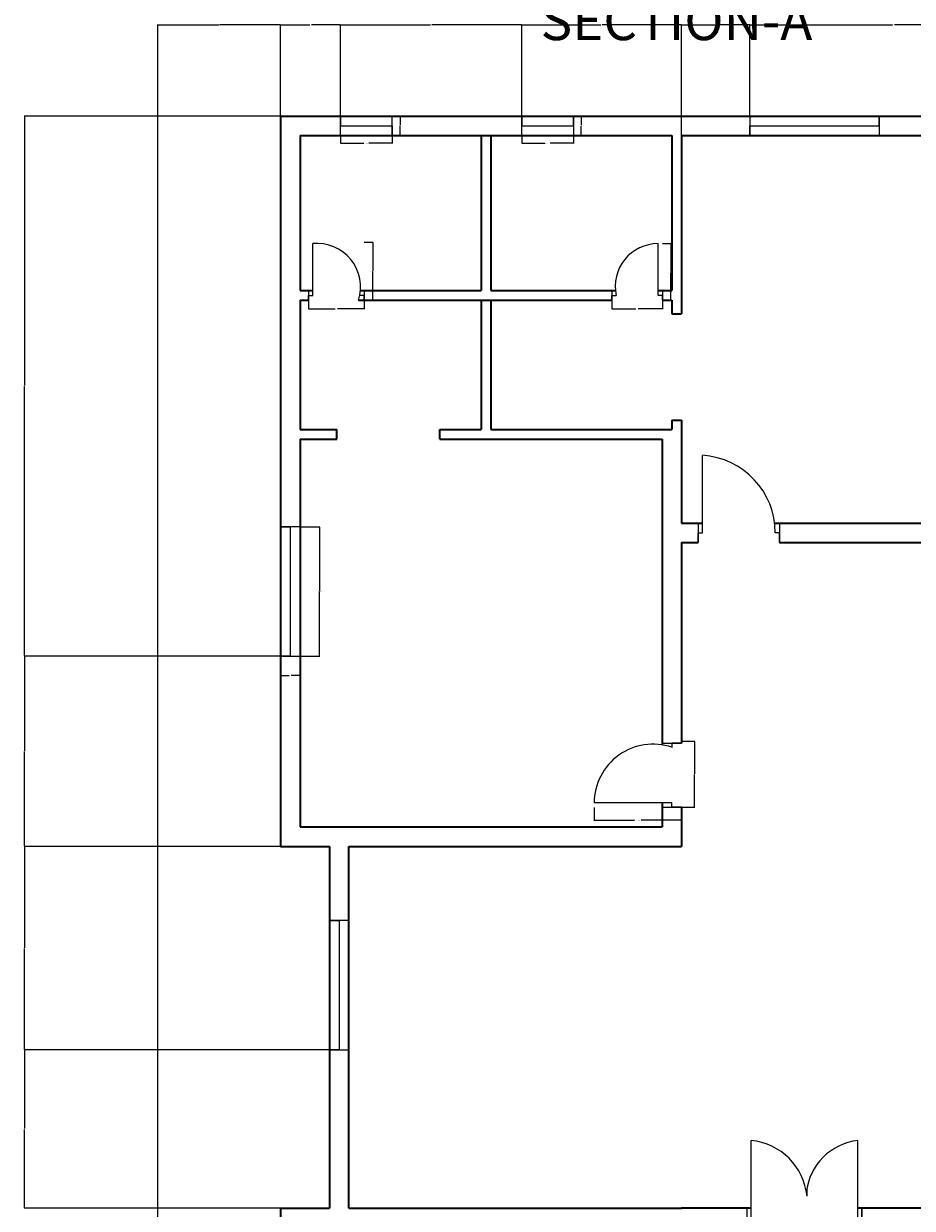
# Model space of a CAD drawing. Units: inches. Extents: x 1824 to 3509, y 619 to 2294.
# Tile 10 of 12: x 2571 to 2983, y 1115 to 1665. Entities that reach past the tile are written whole.
import ezdxf

# ---------------------------------------------------------------- set-up
doc = ezdxf.new("R2010")
doc.units = ezdxf.units.IN
for name, color, linetype, lineweight in [('A-ANNO-DIMS', 2, 'Continuous', 18), ('A-ANNO-TEXT', 7, 'Continuous', 25), ('A-DOOR', 3, 'Continuous', 18), ('A-GLAZ', 4, 'Continuous', 18), ('A-WALL', 7, 'Continuous', 35)]:
    doc.layers.add(name, color=color, linetype=linetype, lineweight=lineweight)
doc.styles.get("Standard").update_dxf_attribs({"font": 'arial.ttf'})
doc.dimstyles.get("Standard").update_dxf_attribs({"dimtxt": 0.18, "dimasz": 0.18, "dimexe": 0.18, "dimexo": 0.0625, "dimgap": 0.09, "dimtad": 0, "dimtih": 1, "dimtoh": 1, "dimdec": 4, "dimzin": 0, "dimdsep": 46, "dimtxsty": 'Standard', "dimcen": 0.09, "dimadec": 0, "dimazin": 0, "dimtfac": 1, "dimtdec": 4, "dimtofl": 0, "dimtmove": 0, "dimatfit": 3, "dimfxl": 1, "dimtolj": 1, "dimtzin": 0, "dimarcsym": 0})

# ---------------------------------------------------------------- blocks, each defined once
blk = doc.blocks.new('DOOR-BATH-W-24')
for p, q in [((2, 2.25), (2, 26.25)), ((0, 4.5), (0, 0)), ((0, 0), (0, 2.25)), ((0, 2.25), (2, 2.25)), ((25.84, 2.25), (23.84, 2.25)), ((25.84, 4.5), (25.84, 0)), ((25.84, 0), (25.84, 2.25))]:
    blk.add_line(p, q)
blk.add_arc((4.03, 6.16), 20.2, 342.2542, 95.7568)
blk = doc.blocks.new('DOOR-BATH-C-24')
for p, q in [((21.44, 2.25), (21.44, 26.25)), ((0, 4.5), (0, 0)), ((0, 0), (0, 2.25)), ((0, 2.25), (2, 2.25)), ((23.44, 2.25), (21.44, 2.25)), ((23.44, 4.5), (23.44, 0)), ((23.44, 0), (23.44, 2.25))]:
    blk.add_line(p, q)
blk.add_arc((21.44, 6.38), 19.87, 90, 191.9846)
blk = doc.blocks.new('DOOR-BED-W-36')
for p, q in [((31.5, 29.8), (40.5, 29.8)), ((40.5, 29.8), (36, 29.8)), ((36, 29.8), (36, 27.8)), ((36, 2), (0, 2)), ((31.5, 0), (31.5, 0)), ((31.5, 0), (40.5, 0)), ((36, 0), (36, 2)), ((40.5, 0), (36, 0)), ((36, 0), (36, 0)), ((40.5, 0), (40.5, 0))]:
    blk.add_line(p, q)
blk.add_arc((27.25, 2), 27.25, 71.2585, 180)
blk = doc.blocks.new('DOOR-BED-C-36')
for p, q in [((2, 4.5), (2, 40.5)), ((0, 9), (0, 0)), ((37.83, 9), (37.83, 9)), ((37.83, 9), (37.83, 0)), ((0, 0), (0, 4.5)), ((0, 4.5), (2, 4.5)), ((37.83, 4.5), (35.83, 4.5)), ((37.83, 0), (37.83, 4.5))]:
    blk.add_line(p, q)
blk.add_arc((-0.24, 4.5), 36.07, 0, 86.4439)
blk = doc.blocks.new('DOOR-LOUNGE-PAIR')
for p, q in [((2, 4.5), (2, 40.5)), ((51.41, 4.5), (51.41, 40.5)), ((27.9, 14.63), (27.9, 18.05)), ((0, 9), (0, 0)), ((53.41, 0), (53.41, 9)), ((53.41, 9), (53.41, 4.5)), ((0, 0), (0, 4.5)), ((0, 4.5), (2, 4.5)), ((53.41, 4.5), (51.41, 4.5)), ((53.41, 4.5), (53.41, 4.5))]:
    blk.add_line(p, q)
for centre, radius, start, end in [((-0.78, 11.81), 28.82, 5.6014, 84.4566), ((54.5, 13.67), 27.01, 96.5732, 173.8895)]:
    blk.add_arc(centre, radius, start, end)
blk = doc.blocks.new('WIN-24')
for p, q in [((0, 0), (0, 9)), ((0, 9), (0, 4.5)), ((24, 0), (24, 9)), ((0, 4.5), (24, 4.5)), ((24, 4.5), (24, 0))]:
    blk.add_line(p, q)
blk = doc.blocks.new('WIN-60')
for p, q in [((0, 9), (0, 0)), ((60, 4.5), (60, 9)), ((60, 9), (60, 0)), ((0, 0), (0, 4.5)), ((0, 4.5), (60, 4.5))]:
    blk.add_line(p, q)
blk = doc.blocks.new('WIN-60-SIDE')
for p, q in [((9, 60), (0, 60)), ((0, 60), (4.5, 60)), ((4.5, 60), (4.5, 0)), ((4.5, 0), (0, 0)), ((0, 0), (9, 0))]:
    blk.add_line(p, q)
blk = doc.blocks.new('WIN-24-TOP')
for p, q in [((0, 0), (0, 9)), ((0, 9), (0, 4.5)), ((24, 4.5), (24, 9)), ((24, 9), (24, 0)), ((0, 4.5), (24, 4.5))]:
    blk.add_line(p, q)
blk = doc.blocks.new('*D32')
at = {"layer": 'A-ANNO-DIMS', "color": 0, "lineweight": -2, "transparency": 16777216}
for p, q in [((2717.54, 1613.04), (2717.54, 1609.32)), ((2741.54, 1613.04), (2741.54, 1609.32)), ((2717.72, 1609.5), (2728.42, 1609.5)), ((2741.36, 1609.5), (2730.65, 1609.5))]:
    blk.add_line(p, q, dxfattribs=at)
at = {"layer": 'A-ANNO-DIMS', "color": 0, "transparency": 16777216}
for points in [[(2717.72, 1609.53), (2717.72, 1609.47), (2717.54, 1609.5)], [(2741.36, 1609.53), (2741.36, 1609.47), (2741.54, 1609.5)]]:
    blk.add_solid(points, dxfattribs=at)
at = {"layer": 'Defpoints', "color": 0, "transparency": 16777216}
for p in [(2717.54, 1613.1), (2741.54, 1613.1), (2741.54, 1609.5)]:
    blk.add_point(p, dxfattribs=at)
at = {"layer": 'A-ANNO-DIMS', "color": 0, "transparency": 16777216, "insert": (2729.54, 1609.5), "char_height": 0.18, "attachment_point": 5}
blk.add_mtext('\\A1;WINDOW 24 TYP.', dxfattribs=at)
blk = doc.blocks.new('*D33')
at = {"layer": 'A-ANNO-DIMS', "color": 0, "lineweight": -2, "transparency": 16777216}
for p, q in [((2741.6, 1622.1), (2745.32, 1622.1)), ((2745.14, 1621.92), (2745.14, 1617.78)), ((2745.14, 1613.28), (2745.14, 1617.42)), ((2741.6, 1613.1), (2745.32, 1613.1))]:
    blk.add_line(p, q, dxfattribs=at)
at = {"layer": 'A-ANNO-DIMS', "color": 0, "transparency": 16777216}
for points in [[(2745.11, 1621.92), (2745.17, 1621.92), (2745.14, 1622.1)], [(2745.11, 1613.28), (2745.17, 1613.28), (2745.14, 1613.1)]]:
    blk.add_solid(points, dxfattribs=at)
at = {"layer": 'Defpoints', "color": 0, "transparency": 16777216}
for p in [(2741.54, 1622.1), (2745.14, 1622.1), (2741.54, 1613.1)]:
    blk.add_point(p, dxfattribs=at)
at = {"layer": 'A-ANNO-DIMS', "color": 0, "transparency": 16777216, "insert": (2745.14, 1617.6), "char_height": 0.18, "attachment_point": 5}
blk.add_mtext('\\A1;9 TYP.', dxfattribs=at)
blk = doc.blocks.new('*D44')
at = {"layer": 'A-ANNO-DIMS', "color": 0, "lineweight": -2, "transparency": 16777216}
for p, q in [((2698.79, 1431.44), (2707.91, 1431.44)), ((2707.73, 1431.26), (2707.73, 1401.62)), ((2707.73, 1371.62), (2707.73, 1401.26)), ((2698.79, 1371.44), (2707.91, 1371.44))]:
    blk.add_line(p, q, dxfattribs=at)
at = {"layer": 'A-ANNO-DIMS', "color": 0, "transparency": 16777216}
for points in [[(2707.7, 1431.26), (2707.76, 1431.26), (2707.73, 1431.44)], [(2707.7, 1371.62), (2707.76, 1371.62), (2707.73, 1371.44)]]:
    blk.add_solid(points, dxfattribs=at)
at = {"layer": 'Defpoints', "color": 0, "transparency": 16777216}
for p in [(2698.73, 1431.44), (2707.73, 1431.44), (2698.73, 1371.44)]:
    blk.add_point(p, dxfattribs=at)
at = {"layer": 'A-ANNO-DIMS', "color": 0, "transparency": 16777216, "insert": (2707.73, 1401.44), "char_height": 0.18, "attachment_point": 5}
blk.add_mtext('\\A1;SIDE WINDOW 60 TYP.', dxfattribs=at)
blk = doc.blocks.new('*D45')
at = {"layer": 'A-ANNO-DIMS', "color": 0, "lineweight": -2, "transparency": 16777216}
for p, q in [((2689.73, 1371.38), (2689.73, 1362.26)), ((2698.73, 1371.38), (2698.73, 1362.26)), ((2689.91, 1362.44), (2693.77, 1362.44)), ((2698.55, 1362.44), (2694.69, 1362.44))]:
    blk.add_line(p, q, dxfattribs=at)
at = {"layer": 'A-ANNO-DIMS', "color": 0, "transparency": 16777216}
for points in [[(2689.91, 1362.47), (2689.91, 1362.41), (2689.73, 1362.44)], [(2698.55, 1362.47), (2698.55, 1362.41), (2698.73, 1362.44)]]:
    blk.add_solid(points, dxfattribs=at)
at = {"layer": 'Defpoints', "color": 0, "transparency": 16777216}
for p in [(2689.73, 1371.44), (2698.73, 1371.44), (2698.73, 1362.44)]:
    blk.add_point(p, dxfattribs=at)
at = {"layer": 'A-ANNO-DIMS', "color": 0, "transparency": 16777216, "insert": (2694.23, 1362.44), "char_height": 0.18, "attachment_point": 5}
blk.add_mtext('\\A1;9 TYP.', dxfattribs=at)
blk = doc.blocks.new('*D56')
at = {"layer": 'A-ANNO-DIMS', "color": 0, "lineweight": -2, "transparency": 16777216}
for p, q in [((2728.54, 1563.53), (2732.69, 1563.53)), ((2732.51, 1563.35), (2732.51, 1550.25)), ((2732.51, 1536.78), (2732.51, 1549.88)), ((2728.54, 1536.6), (2732.69, 1536.6))]:
    blk.add_line(p, q, dxfattribs=at)
at = {"layer": 'A-ANNO-DIMS', "color": 0, "transparency": 16777216}
for points in [[(2732.48, 1563.35), (2732.54, 1563.35), (2732.51, 1563.53)], [(2732.48, 1536.78), (2732.54, 1536.78), (2732.51, 1536.6)]]:
    blk.add_solid(points, dxfattribs=at)
at = {"layer": 'Defpoints', "color": 0, "transparency": 16777216}
for p in [(2728.47, 1563.53), (2732.51, 1563.53), (2728.47, 1536.6)]:
    blk.add_point(p, dxfattribs=at)
at = {"layer": 'A-ANNO-DIMS', "color": 0, "transparency": 16777216, "insert": (2732.51, 1550.07), "char_height": 0.18, "attachment_point": 5}
blk.add_mtext('\\A1;BATH DOOR 27 TYP.', dxfattribs=at)
blk = doc.blocks.new('*D57')
at = {"layer": 'A-ANNO-DIMS', "color": 0, "lineweight": -2, "transparency": 16777216}
for p, q in [((2702.63, 1536.54), (2702.63, 1532.38)), ((2728.47, 1536.54), (2728.47, 1532.38)), ((2702.81, 1532.56), (2715.02, 1532.56)), ((2728.29, 1532.56), (2716.08, 1532.56))]:
    blk.add_line(p, q, dxfattribs=at)
at = {"layer": 'A-ANNO-DIMS', "color": 0, "transparency": 16777216}
for points in [[(2702.81, 1532.59), (2702.81, 1532.53), (2702.63, 1532.56)], [(2728.29, 1532.59), (2728.29, 1532.53), (2728.47, 1532.56)]]:
    blk.add_solid(points, dxfattribs=at)
at = {"layer": 'Defpoints', "color": 0, "transparency": 16777216}
for p in [(2702.63, 1536.6), (2728.47, 1536.6), (2728.47, 1532.56)]:
    blk.add_point(p, dxfattribs=at)
at = {"layer": 'A-ANNO-DIMS', "color": 0, "transparency": 16777216, "insert": (2715.55, 1532.56), "char_height": 0.18, "attachment_point": 5}
blk.add_mtext('\\A1;26 TYP.', dxfattribs=at)
blk = doc.blocks.new('*D58')
at = {"layer": 'A-ANNO-DIMS', "color": 0, "lineweight": -2, "transparency": 16777216}
for p, q in [((2866.92, 1562.85), (2870.97, 1562.85)), ((2870.79, 1562.67), (2870.79, 1549.91)), ((2870.79, 1536.78), (2870.79, 1549.54)), ((2866.92, 1536.6), (2870.97, 1536.6))]:
    blk.add_line(p, q, dxfattribs=at)
at = {"layer": 'A-ANNO-DIMS', "color": 0, "transparency": 16777216}
for points in [[(2870.76, 1562.67), (2870.82, 1562.67), (2870.79, 1562.85)], [(2870.76, 1536.78), (2870.82, 1536.78), (2870.79, 1536.6)]]:
    blk.add_solid(points, dxfattribs=at)
at = {"layer": 'Defpoints', "color": 0, "transparency": 16777216}
for p in [(2866.86, 1562.85), (2870.79, 1562.85), (2866.86, 1536.6)]:
    blk.add_point(p, dxfattribs=at)
at = {"layer": 'A-ANNO-DIMS', "color": 0, "transparency": 16777216, "insert": (2870.79, 1549.73), "char_height": 0.18, "attachment_point": 5}
blk.add_mtext('\\A1;BATH DOOR 26 TYP.', dxfattribs=at)
blk = doc.blocks.new('*D59')
at = {"layer": 'A-ANNO-DIMS', "color": 0, "lineweight": -2, "transparency": 16777216}
for p, q in [((2843.42, 1536.54), (2843.42, 1532.48)), ((2866.86, 1536.54), (2866.86, 1532.48)), ((2843.6, 1532.66), (2854.61, 1532.66)), ((2866.68, 1532.66), (2855.67, 1532.66))]:
    blk.add_line(p, q, dxfattribs=at)
at = {"layer": 'A-ANNO-DIMS', "color": 0, "transparency": 16777216}
for points in [[(2843.6, 1532.69), (2843.6, 1532.63), (2843.42, 1532.66)], [(2866.68, 1532.69), (2866.68, 1532.63), (2866.86, 1532.66)]]:
    blk.add_solid(points, dxfattribs=at)
at = {"layer": 'Defpoints', "color": 0, "transparency": 16777216}
for p in [(2843.42, 1536.6), (2866.86, 1536.6), (2866.86, 1532.66)]:
    blk.add_point(p, dxfattribs=at)
at = {"layer": 'A-ANNO-DIMS', "color": 0, "transparency": 16777216, "insert": (2855.14, 1532.66), "char_height": 0.18, "attachment_point": 5}
blk.add_mtext('\\A1;23 TYP.', dxfattribs=at)
blk = doc.blocks.new('*D60')
at = {"layer": 'A-ANNO-DIMS', "color": 0, "lineweight": -2, "transparency": 16777216}
for p, q in [((2835.23, 1301.2), (2835.23, 1295.01)), ((2875.73, 1301.2), (2875.73, 1295.01)), ((2835.41, 1295.19), (2853.86, 1295.19)), ((2875.55, 1295.19), (2857.1, 1295.19))]:
    blk.add_line(p, q, dxfattribs=at)
at = {"layer": 'A-ANNO-DIMS', "color": 0, "transparency": 16777216}
for points in [[(2835.41, 1295.22), (2835.41, 1295.16), (2835.23, 1295.19)], [(2875.55, 1295.22), (2875.55, 1295.16), (2875.73, 1295.19)]]:
    blk.add_solid(points, dxfattribs=at)
at = {"layer": 'Defpoints', "color": 0, "transparency": 16777216}
for p in [(2835.23, 1301.26), (2875.73, 1301.26), (2875.73, 1295.19)]:
    blk.add_point(p, dxfattribs=at)
at = {"layer": 'A-ANNO-DIMS', "color": 0, "transparency": 16777216, "insert": (2855.48, 1295.19), "char_height": 0.18, "attachment_point": 5}
blk.add_mtext('\\A1;BEDROOM DOOR 41 TYP.', dxfattribs=at)
blk = doc.blocks.new('*D61')
at = {"layer": 'A-ANNO-DIMS', "color": 0, "lineweight": -2, "transparency": 16777216}
for p, q in [((2875.79, 1331.89), (2881.98, 1331.89)), ((2881.8, 1331.71), (2881.8, 1316.76)), ((2881.8, 1301.44), (2881.8, 1316.39)), ((2875.79, 1301.26), (2881.98, 1301.26))]:
    blk.add_line(p, q, dxfattribs=at)
at = {"layer": 'A-ANNO-DIMS', "color": 0, "transparency": 16777216}
for points in [[(2881.77, 1331.71), (2881.83, 1331.71), (2881.8, 1331.89)], [(2881.77, 1301.44), (2881.83, 1301.44), (2881.8, 1301.26)]]:
    blk.add_solid(points, dxfattribs=at)
at = {"layer": 'Defpoints', "color": 0, "transparency": 16777216}
for p in [(2875.73, 1331.89), (2881.8, 1331.89), (2875.73, 1301.26)]:
    blk.add_point(p, dxfattribs=at)
at = {"layer": 'A-ANNO-DIMS', "color": 0, "transparency": 16777216, "insert": (2881.8, 1316.58), "char_height": 0.18, "attachment_point": 5}
blk.add_mtext('\\A1;31 TYP.', dxfattribs=at)
blk = doc.blocks.new('*D84')
at = {"layer": 'A-ANNO-DIMS', "color": 0, "lineweight": -2, "transparency": 16777216}
for p, q in [((2801.63, 1613.04), (2801.63, 1609.32)), ((2825.63, 1613.04), (2825.63, 1609.32)), ((2801.81, 1609.5), (2812.52, 1609.5)), ((2825.45, 1609.5), (2814.75, 1609.5))]:
    blk.add_line(p, q, dxfattribs=at)
at = {"layer": 'A-ANNO-DIMS', "color": 0, "transparency": 16777216}
for points in [[(2801.81, 1609.53), (2801.81, 1609.47), (2801.63, 1609.5)], [(2825.45, 1609.53), (2825.45, 1609.47), (2825.63, 1609.5)]]:
    blk.add_solid(points, dxfattribs=at)
at = {"layer": 'Defpoints', "color": 0, "transparency": 16777216}
for p in [(2801.63, 1613.1), (2825.63, 1613.1), (2825.63, 1609.5)]:
    blk.add_point(p, dxfattribs=at)
at = {"layer": 'A-ANNO-DIMS', "color": 0, "transparency": 16777216, "insert": (2813.63, 1609.5), "char_height": 0.18, "attachment_point": 5}
blk.add_mtext('\\A1;WINDOW 24 TYP.', dxfattribs=at)
blk = doc.blocks.new('*D85')
at = {"layer": 'A-ANNO-DIMS', "color": 0, "lineweight": -2, "transparency": 16777216}
for p, q in [((2825.7, 1622.1), (2829.41, 1622.1)), ((2829.23, 1621.92), (2829.23, 1617.78)), ((2829.23, 1613.28), (2829.23, 1617.42)), ((2825.7, 1613.1), (2829.41, 1613.1))]:
    blk.add_line(p, q, dxfattribs=at)
at = {"layer": 'A-ANNO-DIMS', "color": 0, "transparency": 16777216}
for points in [[(2829.2, 1621.92), (2829.26, 1621.92), (2829.23, 1622.1)], [(2829.2, 1613.28), (2829.26, 1613.28), (2829.23, 1613.1)]]:
    blk.add_solid(points, dxfattribs=at)
at = {"layer": 'Defpoints', "color": 0, "transparency": 16777216}
for p in [(2825.63, 1622.1), (2829.23, 1622.1), (2825.63, 1613.1)]:
    blk.add_point(p, dxfattribs=at)
at = {"layer": 'A-ANNO-DIMS', "color": 0, "transparency": 16777216, "insert": (2829.23, 1617.6), "char_height": 0.18, "attachment_point": 5}
blk.add_mtext('\\A1;9 TYP.', dxfattribs=at)
blk = doc.blocks.new('*D104')
at = {"layer": 'A-ANNO-DIMS', "color": 0, "lineweight": -2, "transparency": 16777216}
for p, q in [((3206.79, 1622.1), (3329.93, 1622.1)), ((3329.75, 1621.92), (3329.75, 1202.28)), ((3329.75, 782.28), (3329.75, 1201.92)), ((2875.79, 782.1), (3329.93, 782.1))]:
    blk.add_line(p, q, dxfattribs=at)
at = {"layer": 'A-ANNO-DIMS', "color": 0, "transparency": 16777216}
for points in [[(3329.72, 1621.92), (3329.78, 1621.92), (3329.75, 1622.1)], [(3329.72, 782.28), (3329.78, 782.28), (3329.75, 782.1)]]:
    blk.add_solid(points, dxfattribs=at)
at = {"layer": 'Defpoints', "color": 0, "transparency": 16777216}
for p in [(3206.73, 1622.1), (3329.75, 1622.1), (2875.73, 782.1)]:
    blk.add_point(p, dxfattribs=at)
at = {"layer": 'A-ANNO-DIMS', "color": 0, "transparency": 16777216, "insert": (3329.75, 1202.1), "char_height": 0.18, "attachment_point": 5}
blk.add_mtext('\\A1;840', dxfattribs=at)
blk = doc.blocks.new('*D107')
at = {"layer": 'A-ANNO-DIMS', "color": 0, "lineweight": -2, "transparency": 16777216}
for p, q in [((2712.28, 1188.68), (2570.72, 1188.68)), ((2570.9, 1188.5), (2570.9, 1152.07)), ((2570.9, 1115.28), (2570.9, 1151.71)), ((2689.67, 1115.1), (2570.72, 1115.1))]:
    blk.add_line(p, q, dxfattribs=at)
at = {"layer": 'A-ANNO-DIMS', "color": 0, "transparency": 16777216}
for points in [[(2570.87, 1188.5), (2570.93, 1188.5), (2570.9, 1188.68)], [(2570.87, 1115.28), (2570.93, 1115.28), (2570.9, 1115.1)]]:
    blk.add_solid(points, dxfattribs=at)
at = {"layer": 'Defpoints', "color": 0, "transparency": 16777216}
for p in [(2570.9, 1188.68), (2712.34, 1188.68), (2689.73, 1115.1)]:
    blk.add_point(p, dxfattribs=at)
at = {"layer": 'A-ANNO-DIMS', "color": 0, "transparency": 16777216, "insert": (2570.9, 1151.89), "char_height": 0.18, "attachment_point": 5}
blk.add_mtext('\\A1;73.58', dxfattribs=at)
blk = doc.blocks.new('*D108')
at = {"layer": 'A-ANNO-DIMS', "color": 0, "lineweight": -2, "transparency": 16777216}
for p, q in [((2689.67, 1283.1), (2570.72, 1283.1)), ((2570.9, 1282.92), (2570.9, 1236.07)), ((2570.9, 1188.86), (2570.9, 1235.71)), ((2712.28, 1188.68), (2570.72, 1188.68))]:
    blk.add_line(p, q, dxfattribs=at)
at = {"layer": 'A-ANNO-DIMS', "color": 0, "transparency": 16777216}
for points in [[(2570.87, 1282.92), (2570.93, 1282.92), (2570.9, 1283.1)], [(2570.87, 1188.86), (2570.93, 1188.86), (2570.9, 1188.68)]]:
    blk.add_solid(points, dxfattribs=at)
at = {"layer": 'Defpoints', "color": 0, "transparency": 16777216}
for p in [(2570.9, 1283.1), (2689.73, 1283.1), (2712.34, 1188.68)]:
    blk.add_point(p, dxfattribs=at)
at = {"layer": 'A-ANNO-DIMS', "color": 0, "transparency": 16777216, "insert": (2570.9, 1235.89), "char_height": 0.18, "attachment_point": 5}
blk.add_mtext('\\A1;94.42', dxfattribs=at)
blk = doc.blocks.new('*D109')
at = {"layer": 'A-ANNO-DIMS', "color": 0, "lineweight": -2, "transparency": 16777216}
for p, q in [((2689.67, 1371.44), (2570.72, 1371.44)), ((2570.9, 1371.26), (2570.9, 1327.45)), ((2570.9, 1283.28), (2570.9, 1327.09)), ((2689.67, 1283.1), (2570.72, 1283.1))]:
    blk.add_line(p, q, dxfattribs=at)
at = {"layer": 'A-ANNO-DIMS', "color": 0, "transparency": 16777216}
for points in [[(2570.87, 1371.26), (2570.93, 1371.26), (2570.9, 1371.44)], [(2570.87, 1283.28), (2570.93, 1283.28), (2570.9, 1283.1)]]:
    blk.add_solid(points, dxfattribs=at)
at = {"layer": 'Defpoints', "color": 0, "transparency": 16777216}
for p in [(2570.9, 1371.44), (2689.73, 1371.44), (2689.73, 1283.1)]:
    blk.add_point(p, dxfattribs=at)
at = {"layer": 'A-ANNO-DIMS', "color": 0, "transparency": 16777216, "insert": (2570.9, 1327.27), "char_height": 0.18, "attachment_point": 5}
blk.add_mtext('\\A1;88.34', dxfattribs=at)
blk = doc.blocks.new('*D110')
at = {"layer": 'A-ANNO-DIMS', "color": 0, "lineweight": -2, "transparency": 16777216}
for p, q in [((2689.67, 1622.1), (2570.72, 1622.1)), ((2570.9, 1621.92), (2570.9, 1496.95)), ((2570.9, 1371.62), (2570.9, 1496.59)), ((2689.67, 1371.44), (2570.72, 1371.44))]:
    blk.add_line(p, q, dxfattribs=at)
at = {"layer": 'A-ANNO-DIMS', "color": 0, "transparency": 16777216}
for points in [[(2570.87, 1621.92), (2570.93, 1621.92), (2570.9, 1622.1)], [(2570.87, 1371.62), (2570.93, 1371.62), (2570.9, 1371.44)]]:
    blk.add_solid(points, dxfattribs=at)
at = {"layer": 'Defpoints', "color": 0, "transparency": 16777216}
for p in [(2570.9, 1622.1), (2689.73, 1622.1), (2689.73, 1371.44)]:
    blk.add_point(p, dxfattribs=at)
at = {"layer": 'A-ANNO-DIMS', "color": 0, "transparency": 16777216, "insert": (2570.9, 1496.77), "char_height": 0.18, "attachment_point": 5}
blk.add_mtext('\\A1;250.66', dxfattribs=at)
blk = doc.blocks.new('*D111')
at = {"layer": 'A-ANNO-DIMS', "color": 0, "lineweight": -2, "transparency": 16777216}
for p, q in [((2632.73, 1049.16), (2632.73, 1664.63)), ((2632.91, 1664.45), (2661.01, 1664.45)), ((2689.55, 1664.45), (2661.45, 1664.45)), ((2689.73, 1283.16), (2689.73, 1664.63))]:
    blk.add_line(p, q, dxfattribs=at)
at = {"layer": 'A-ANNO-DIMS', "color": 0, "transparency": 16777216}
for points in [[(2632.91, 1664.48), (2632.91, 1664.42), (2632.73, 1664.45)], [(2689.55, 1664.48), (2689.55, 1664.42), (2689.73, 1664.45)]]:
    blk.add_solid(points, dxfattribs=at)
at = {"layer": 'Defpoints', "color": 0, "transparency": 16777216}
for p in [(2632.73, 1664.45), (2689.73, 1283.1), (2632.73, 1049.1)]:
    blk.add_point(p, dxfattribs=at)
at = {"layer": 'A-ANNO-DIMS', "color": 0, "transparency": 16777216, "insert": (2661.23, 1664.45), "char_height": 0.18, "attachment_point": 5}
blk.add_mtext('\\A1;57', dxfattribs=at)
blk = doc.blocks.new('*D112')
at = {"layer": 'A-ANNO-DIMS', "color": 0, "lineweight": -2, "transparency": 16777216}
for p, q in [((2689.73, 1622.16), (2689.73, 1664.63)), ((2689.91, 1664.45), (2703.25, 1664.45)), ((2717.36, 1664.45), (2704.01, 1664.45)), ((2717.54, 1622.16), (2717.54, 1664.63))]:
    blk.add_line(p, q, dxfattribs=at)
at = {"layer": 'A-ANNO-DIMS', "color": 0, "transparency": 16777216}
for points in [[(2689.91, 1664.48), (2689.91, 1664.42), (2689.73, 1664.45)], [(2717.36, 1664.48), (2717.36, 1664.42), (2717.54, 1664.45)]]:
    blk.add_solid(points, dxfattribs=at)
at = {"layer": 'Defpoints', "color": 0, "transparency": 16777216}
for p in [(2717.54, 1664.45), (2689.73, 1622.1), (2717.54, 1622.1)]:
    blk.add_point(p, dxfattribs=at)
at = {"layer": 'A-ANNO-DIMS', "color": 0, "transparency": 16777216, "insert": (2703.63, 1664.45), "char_height": 0.18, "attachment_point": 5}
blk.add_mtext('\\A1;27.81', dxfattribs=at)
blk = doc.blocks.new('*D113')
at = {"layer": 'A-ANNO-DIMS', "color": 0, "lineweight": -2, "transparency": 16777216}
for p, q in [((2717.54, 1622.16), (2717.54, 1664.63)), ((2717.72, 1664.45), (2759.28, 1664.45)), ((2801.45, 1664.45), (2759.89, 1664.45)), ((2801.63, 1622.16), (2801.63, 1664.63))]:
    blk.add_line(p, q, dxfattribs=at)
at = {"layer": 'A-ANNO-DIMS', "color": 0, "transparency": 16777216}
for points in [[(2717.72, 1664.48), (2717.72, 1664.42), (2717.54, 1664.45)], [(2801.45, 1664.48), (2801.45, 1664.42), (2801.63, 1664.45)]]:
    blk.add_solid(points, dxfattribs=at)
at = {"layer": 'Defpoints', "color": 0, "transparency": 16777216}
for p in [(2801.63, 1664.45), (2717.54, 1622.1), (2801.63, 1622.1)]:
    blk.add_point(p, dxfattribs=at)
at = {"layer": 'A-ANNO-DIMS', "color": 0, "transparency": 16777216, "insert": (2759.58, 1664.45), "char_height": 0.18, "attachment_point": 5}
blk.add_mtext('\\A1;84.1', dxfattribs=at)
blk = doc.blocks.new('*D114')
at = {"layer": 'A-ANNO-DIMS', "color": 0, "lineweight": -2, "transparency": 16777216}
for p, q in [((2801.63, 1622.16), (2801.63, 1664.63)), ((2801.81, 1664.45), (2838.38, 1664.45)), ((2875.55, 1664.45), (2838.99, 1664.45)), ((2875.73, 1613.16), (2875.73, 1664.63))]:
    blk.add_line(p, q, dxfattribs=at)
at = {"layer": 'A-ANNO-DIMS', "color": 0, "transparency": 16777216}
for points in [[(2801.81, 1664.48), (2801.81, 1664.42), (2801.63, 1664.45)], [(2875.55, 1664.48), (2875.55, 1664.42), (2875.73, 1664.45)]]:
    blk.add_solid(points, dxfattribs=at)
at = {"layer": 'Defpoints', "color": 0, "transparency": 16777216}
for p in [(2875.73, 1664.45), (2801.63, 1622.1), (2875.73, 1613.1)]:
    blk.add_point(p, dxfattribs=at)
at = {"layer": 'A-ANNO-DIMS', "color": 0, "transparency": 16777216, "insert": (2838.68, 1664.45), "char_height": 0.18, "attachment_point": 5}
blk.add_mtext('\\A1;74.1', dxfattribs=at)
blk = doc.blocks.new('*D115')
at = {"layer": 'A-ANNO-DIMS', "color": 0, "lineweight": -2, "transparency": 16777216}
for p, q in [((2875.73, 1613.16), (2875.73, 1664.63)), ((2875.91, 1664.45), (2891.22, 1664.45)), ((2907.32, 1664.45), (2892.01, 1664.45)), ((2907.5, 1622.16), (2907.5, 1664.63))]:
    blk.add_line(p, q, dxfattribs=at)
at = {"layer": 'A-ANNO-DIMS', "color": 0, "transparency": 16777216}
for points in [[(2875.91, 1664.48), (2875.91, 1664.42), (2875.73, 1664.45)], [(2907.32, 1664.48), (2907.32, 1664.42), (2907.5, 1664.45)]]:
    blk.add_solid(points, dxfattribs=at)
at = {"layer": 'Defpoints', "color": 0, "transparency": 16777216}
for p in [(2907.5, 1664.45), (2907.5, 1622.1), (2875.73, 1613.1)]:
    blk.add_point(p, dxfattribs=at)
at = {"layer": 'A-ANNO-DIMS', "color": 0, "transparency": 16777216, "insert": (2891.61, 1664.45), "char_height": 0.18, "attachment_point": 5}
blk.add_mtext('\\A1;31.77', dxfattribs=at)
blk = doc.blocks.new('*D116')
at = {"layer": 'A-ANNO-DIMS', "color": 0, "lineweight": -2, "transparency": 16777216}
for p, q in [((2907.5, 1622.16), (2907.5, 1664.63)), ((2907.68, 1664.45), (2973.66, 1664.45)), ((3040.55, 1664.45), (2974.57, 1664.45)), ((3040.73, 1613.16), (3040.73, 1664.63))]:
    blk.add_line(p, q, dxfattribs=at)
at = {"layer": 'A-ANNO-DIMS', "color": 0, "transparency": 16777216}
for points in [[(2907.68, 1664.48), (2907.68, 1664.42), (2907.5, 1664.45)], [(3040.55, 1664.48), (3040.55, 1664.42), (3040.73, 1664.45)]]:
    blk.add_solid(points, dxfattribs=at)
at = {"layer": 'Defpoints', "color": 0, "transparency": 16777216}
for p in [(3040.73, 1664.45), (2907.5, 1622.1), (3040.73, 1613.1)]:
    blk.add_point(p, dxfattribs=at)
at = {"layer": 'A-ANNO-DIMS', "color": 0, "transparency": 16777216, "insert": (2974.11, 1664.45), "char_height": 0.18, "attachment_point": 5}
blk.add_mtext('\\A1;133.23', dxfattribs=at)

msp = doc.modelspace()

# ---------------------------------------------------------------- linework, layer by layer
at = {"layer": 'A-GLAZ'}
msp.add_line((2801.6339, 1622.1012), (2801.6339, 1622.1012), dxfattribs=at)
at = {"layer": 'A-WALL'}
for p, q in [((2689.7282, 1622.1012), (2689.7282, 1283.1012)), ((2689.7282, 1622.1012), (3206.7282, 1622.1012)), ((2698.7282, 1613.1012), (2698.7282, 1541.1012)), ((2698.7282, 1613.1012), (2871.2282, 1613.1012)), ((2782.7282, 1613.1012), (2782.7282, 1541.1012)), ((2787.2282, 1613.1012), (2787.2282, 1541.1012)), ((2871.2282, 1613.1012), (2871.2282, 1541.1012)), ((2875.7282, 1613.1012), (2875.7282, 1536.6012)), ((2875.7282, 1613.1012), (3031.7282, 1613.1012)), ((2698.7282, 1541.1012), (2704.6333, 1541.1012)), ((2726.7873, 1541.1012), (2782.7282, 1541.1012)), ((2787.2282, 1541.1012), (2845.0729, 1541.1012)), ((2864.8574, 1541.1012), (2871.2282, 1541.1012)), ((2698.7282, 1536.6012), (2698.7282, 1476.6012)), ((2698.7282, 1536.6012), (2702.6333, 1536.6012)), ((2725.8943, 1536.6012), (2843.4173, 1536.6012)), ((2782.7282, 1536.6012), (2782.7282, 1476.6012)), ((2787.2282, 1536.6012), (2787.2282, 1476.6012)), ((2866.8574, 1536.6012), (2871.2282, 1536.6012)), ((2871.2282, 1536.6012), (2871.2282, 1530.3011)), ((2875.7282, 1536.6012), (2875.7282, 1530.3011)), ((2871.2282, 1530.3011), (2871.2282, 1530.3011)), ((2871.2282, 1530.3011), (2875.7282, 1530.3011)), ((2871.2282, 1480.9642), (2871.2282, 1476.6012)), ((2871.2282, 1480.9642), (2875.7282, 1480.9642)), ((2875.7282, 1480.9642), (2875.7282, 1433.1012)), ((2698.7282, 1476.6012), (2715.782, 1476.6012)), ((2715.782, 1472.1012), (2715.782, 1476.6012)), ((2763.6589, 1476.6012), (2782.7282, 1476.6012)), ((2763.6589, 1472.1012), (2763.6589, 1476.6012)), ((2787.2282, 1476.6012), (2871.2282, 1476.6012)), ((2698.7282, 1472.1012), (2698.7282, 1292.1012)), ((2698.7282, 1472.1012), (2715.782, 1472.1012)), ((2715.782, 1472.1012), (2715.782, 1472.1012)), ((2763.6589, 1472.1012), (2866.7282, 1472.1012)), ((2866.7282, 1472.1012), (2866.7282, 1330.1752)), ((2875.7282, 1433.1012), (2885.4395, 1433.1012)), ((2918.9899, 1433.1012), (3031.7282, 1433.1012)), ((2875.7282, 1424.1012), (2875.7282, 1331.0647)), ((2875.7282, 1424.1012), (2883.4395, 1424.1012)), ((2921.2717, 1424.1012), (3031.7282, 1424.1012)), ((2866.7282, 1303.2634), (2866.7282, 1292.1012)), ((2875.7282, 1301.2634), (2875.7282, 1283.1012)), ((2698.7282, 1292.1012), (2866.7282, 1292.1012)), ((2689.7282, 1283.1012), (2712.3386, 1283.1012)), ((2712.3386, 1283.1012), (2712.3386, 1115.1012)), ((2721.3386, 1283.1012), (2875.7282, 1283.1012)), ((2721.3386, 1115.1012), (2721.3386, 1283.1012)), ((2689.7282, 1115.1012), (2689.7282, 1049.1012)), ((2689.7282, 1115.1012), (2712.3386, 1115.1012)), ((2721.3386, 1115.1012), (2875.7282, 1115.1012)), ((2721.3386, 1115.1012), (2721.3386, 1115.1012)), ((2908.0784, 1115.1012), (2875.7282, 1115.1012)), ((2992.2282, 1115.1012), (2957.4861, 1115.1012))]:
    msp.add_line(p, q, dxfattribs=at)

# ---------------------------------------------------------------- block references
at = {"layer": 'A-DOOR'}
for name, p in [('DOOR-BATH-W-24', (2702.6333, 1536.601)), ('DOOR-BATH-C-24', (2843.4173, 1536.601)), ('DOOR-BED-C-36', (2883.4393, 1424.101)), ('DOOR-BED-W-36', (2835.2283, 1301.263)), ('DOOR-LOUNGE-PAIR', (2906.0783, 1106.101))]:
    msp.add_blockref(name, p, dxfattribs=at)
at = {"layer": 'A-GLAZ'}
for name, p in [('WIN-24', (2717.5353, 1613.101)), ('WIN-24-TOP', (2801.6343, 1613.101)), ('WIN-60', (2907.4973, 1613.101)), ('WIN-60-SIDE', (2689.7283, 1371.438)), ('WIN-60-SIDE', (2712.3387, 1188.6771))]:
    msp.add_blockref(name, p, dxfattribs=at)

# ---------------------------------------------------------------- texts
at = {"layer": 'A-ANNO-TEXT', "insert": (2810.3821, 1675.3119), "char_height": 18, "attachment_point": 1}
msp.add_mtext_dynamic_manual_height_columns('SECTION-A', width=244.115567, gutter_width=12.5, heights=[0], dxfattribs=at)

# ---------------------------------------------------------------- dimensions: what is measured, and where the dimension line sits
at = {"layer": 'A-ANNO-DIMS'}
for base, p1, p2, override, picture, middle in [((2632.7282, 1664.4512), (2689.7282, 1283.1012), (2632.7282, 1049.1012), {"dimdec": 0, "dimlfac": 1, "dimrnd": 0, "dimzin": 0, "dimdsep": 46, "dimlunit": 2}, '*D111', (2661.2282, 1664.4512)), ((2717.5357, 1664.4512), (2689.7282, 1622.1012), (2717.5357, 1622.1012), {"dimdec": 2, "dimlfac": 1, "dimrnd": 0, "dimzin": 0, "dimdsep": 46, "dimlunit": 2}, '*D112', (2703.6319, 1664.4512)), ((2801.6339, 1664.4512), (2717.5357, 1622.1012), (2801.6339, 1622.1012), {"dimdec": 1, "dimlfac": 1, "dimrnd": 0, "dimzin": 0, "dimdsep": 46, "dimlunit": 2}, '*D113', (2759.5848, 1664.4512)), ((2875.7282, 1664.4512), (2801.6339, 1622.1012), (2875.7282, 1613.1012), {"dimdec": 1, "dimlfac": 1, "dimrnd": 0, "dimzin": 0, "dimdsep": 46, "dimlunit": 2}, '*D114', (2838.6811, 1664.4512)), ((2907.4978, 1664.4512), (2875.7282, 1613.1012), (2907.4978, 1622.1012), {"dimdec": 2, "dimlfac": 1, "dimrnd": 0, "dimzin": 0, "dimdsep": 46, "dimlunit": 2}, '*D115', (2891.613, 1664.4512)), ((3040.7282, 1664.4512), (2907.4978, 1622.1012), (3040.7282, 1613.1012), {"dimdec": 2, "dimlfac": 1, "dimrnd": 0, "dimzin": 0, "dimdsep": 46, "dimlunit": 2}, '*D116', (2974.113, 1664.4512))]:
    dim = msp.add_linear_dim(base=base, p1=p1, p2=p2, dimstyle='Standard', override=override, dxfattribs=at)
    dim.commit()
    dim.dimension.update_dxf_attribs({"geometry": picture, "text_midpoint": middle})
for base, p1, p2, override, picture, middle in [((2570.8984, 1622.1012), (2689.7282, 1371.4382), (2689.7282, 1622.1012), {"dimdec": 2, "dimlfac": 1, "dimrnd": 0, "dimzin": 0, "dimdsep": 46, "dimlunit": 2}, '*D110', (2570.8984, 1496.7697)), ((3329.7513, 1622.1012), (2875.7282, 782.1012), (3206.7282, 1622.1012), {"dimdec": 0, "dimlfac": 1, "dimrnd": 0, "dimzin": 0, "dimdsep": 46, "dimlunit": 2}, '*D104', (3329.7513, 1202.1012)), ((2570.8984, 1371.4382), (2689.7282, 1283.1012), (2689.7282, 1371.4382), {"dimdec": 2, "dimlfac": 1, "dimrnd": 0, "dimzin": 0, "dimdsep": 46, "dimlunit": 2}, '*D109', (2570.8984, 1327.2697)), ((2570.8984, 1283.1012), (2712.3386, 1188.6773), (2689.7282, 1283.1012), {"dimdec": 2, "dimlfac": 1, "dimrnd": 0, "dimzin": 0, "dimdsep": 46, "dimlunit": 2}, '*D108', (2570.8984, 1235.8892)), ((2570.8984, 1188.6773), (2689.7282, 1115.1012), (2712.3386, 1188.6773), {"dimdec": 2, "dimlfac": 1, "dimrnd": 0, "dimzin": 0, "dimdsep": 46, "dimlunit": 2}, '*D107', (2570.8984, 1151.8892))]:
    dim = msp.add_linear_dim(base=base, p1=p1, p2=p2, angle=90, dimstyle='Standard', override=override, dxfattribs=at)
    dim.commit()
    dim.dimension.update_dxf_attribs({"geometry": picture, "text_midpoint": middle})
for base, p1, p2, text, picture, middle in [((2745.1357, 1622.1012), (2741.5357, 1613.1012), (2741.5357, 1622.1012), '<> TYP.', '*D33', (2745.1357, 1617.6012)), ((2829.2339, 1622.1012), (2825.6339, 1613.1012), (2825.6339, 1622.1012), '<> TYP.', '*D85', (2829.2339, 1617.6012)), ((2732.514, 1563.534), (2728.4741, 1536.6012), (2728.4741, 1563.534), 'BATH DOOR <> TYP.', '*D56', (2732.514, 1550.0676)), ((2870.7949, 1562.8512), (2866.8574, 1536.6012), (2866.8574, 1562.8512), 'BATH DOOR <> TYP.', '*D58', (2870.7949, 1549.7262)), ((2707.7282, 1431.4382), (2698.7282, 1371.4382), (2698.7282, 1431.4382), 'SIDE WINDOW <> TYP.', '*D44', (2707.7282, 1401.4382)), ((2881.8032, 1331.8869), (2875.7282, 1301.2634), (2875.7282, 1331.8869), '<> TYP.', '*D61', (2881.8032, 1316.5752))]:
    dim = msp.add_linear_dim(base=base, p1=p1, p2=p2, angle=90, text=text, dimstyle='Standard', override={"dimdec": 0, "dimlfac": 1, "dimrnd": 0, "dimzin": 0, "dimdsep": 46, "dimlunit": 2}, dxfattribs=at)
    dim.commit()
    dim.dimension.update_dxf_attribs({"geometry": picture, "text_midpoint": middle})
for base, p1, p2, text, picture, middle in [((2741.5357, 1609.5012), (2717.5357, 1613.1012), (2741.5357, 1613.1012), 'WINDOW <> TYP.', '*D32', (2729.5357, 1609.5012)), ((2825.6339, 1609.5012), (2801.6339, 1613.1012), (2825.6339, 1613.1012), 'WINDOW <> TYP.', '*D84', (2813.6339, 1609.5012)), ((2728.4741, 1532.5612), (2702.6333, 1536.6012), (2728.4741, 1536.6012), '<> TYP.', '*D57', (2715.5537, 1532.5612)), ((2866.8574, 1532.6637), (2843.4173, 1536.6012), (2866.8574, 1536.6012), '<> TYP.', '*D59', (2855.1374, 1532.6637)), ((2698.7282, 1362.4382), (2689.7282, 1371.4382), (2698.7282, 1371.4382), '<> TYP.', '*D45', (2694.2282, 1362.4382)), ((2875.7282102324, 1295.1884439723), (2835.2282102324, 1301.2634439723), (2875.7282102324, 1301.2634439723), 'BEDROOM DOOR <> TYP.', '*D60', (2855.4782102324, 1295.1884439723))]:
    dim = msp.add_linear_dim(base=base, p1=p1, p2=p2, text=text, dimstyle='Standard', override={"dimdec": 0, "dimlfac": 1, "dimrnd": 0, "dimzin": 0, "dimdsep": 46, "dimlunit": 2}, dxfattribs=at)
    dim.commit()
    dim.dimension.update_dxf_attribs({"geometry": picture, "text_midpoint": middle})

doc.saveas('drawing.dxf')
